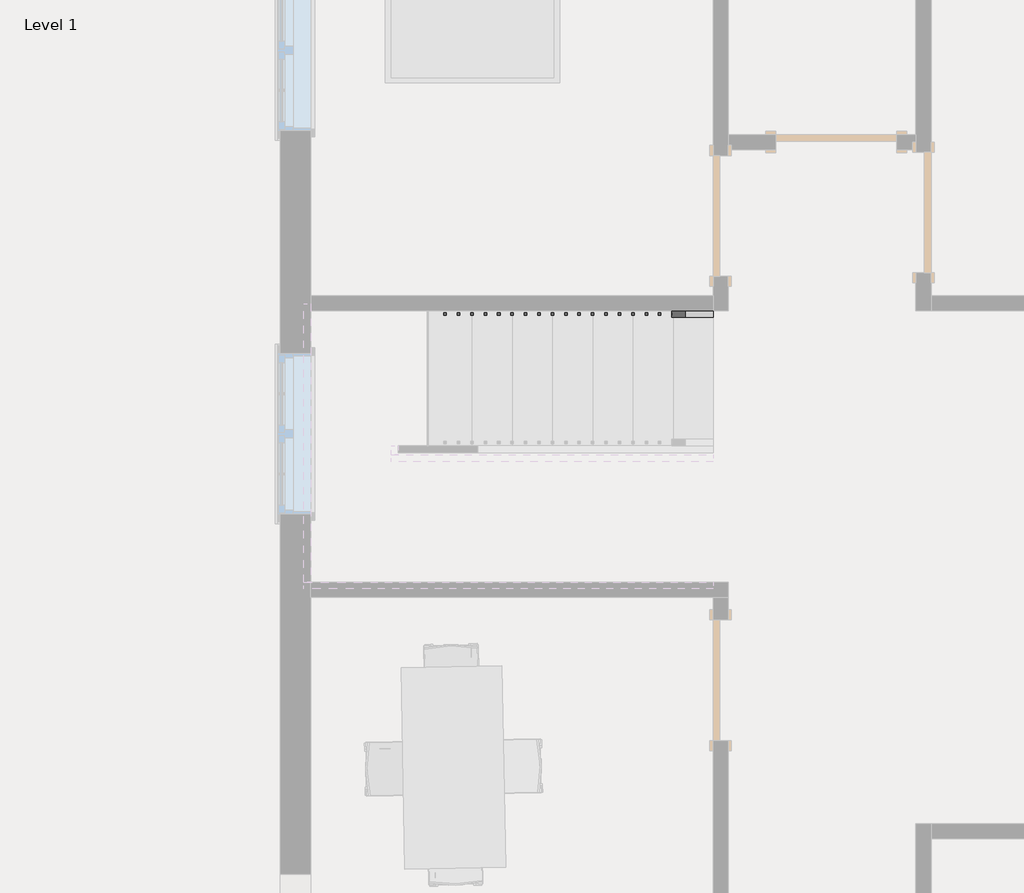
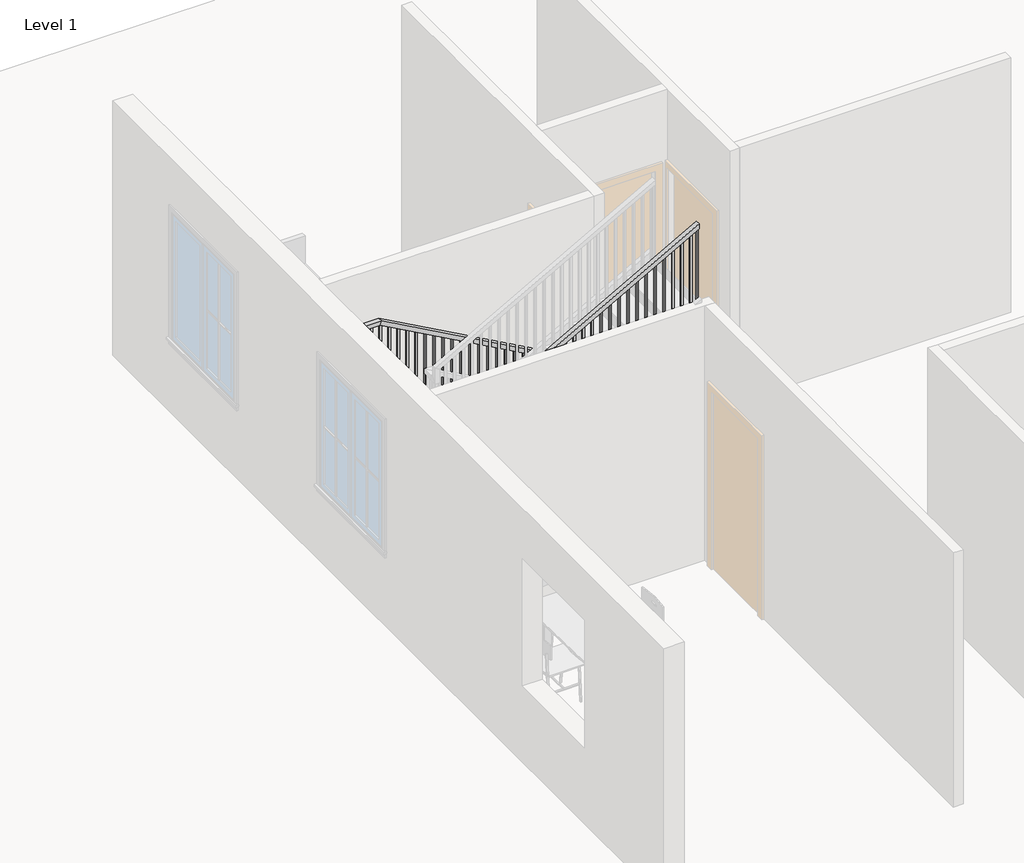
# One storey, part 2 of 3: 1 railing.
"""IFC4 building model written with IfcOpenShell, lengths in millimetres."""

from ifc_helpers import new_model, si_unit, frame, origin, place, context, project, spatial, polyline, outline, extrude, faceted_brep, element, save

model = new_model("IFC4")

# Units and contexts
model_context = context("Model", 3, world=origin())
ifc_project = project(units=[si_unit("LENGTHUNIT", "METRE", prefix="MILLI")], contexts=[model_context])

# Site, building, storey
site = spatial("IfcSite", under=ifc_project)
building = spatial("IfcBuilding", under=site)
storey = spatial("IfcBuildingStorey", under=building, Name="Level 1", Elevation=0.0)

# Railing
placement = place(None, origin())
element("IfcRailing", 1, ObjectType="Handrail - Rectangular", at=placement, inside=storey, context=model_context, shape_type="SolidModel", body=[
    faceted_brep([(4295.1355783, 9918.7, 1083.7333333), (4295.1355783, 9918.7, 1025.620221), (4295.1355783, 9969.5, 1025.620221), (4295.1355783, 9969.5, 1083.7333333), (1856.7355783, 9918.7, 2438.4), (1843.5719761, 9918.7, 2387.6), (1843.5719761, 9969.5, 2387.6), (1856.7355783, 9969.5, 2438.4), (1295.4, 9918.7, 2438.4), (1295.4, 9918.7, 2387.6), (1244.6, 9969.5, 2387.6), (1244.6, 9969.5, 2438.4), (1295.4, 7962.9, 2438.4), (1295.4, 7962.9, 2387.6), (1244.6, 7912.1, 2387.6), (1244.6, 7912.1, 2438.4), (1551.9355783, 7962.9, 2438.4), (1565.0991806, 7962.9, 2387.6), (1565.0991806, 7912.1, 2387.6), (1551.9355783, 7912.1, 2438.4), (4295.1355783, 7962.9, 3962.4), (4295.1355783, 7912.1, 3962.4), (4295.1355783, 7912.1, 3904.2868876), (4295.1355783, 7962.9, 3904.2868876)], [[[0, 1, 2, 3]], [[1, 0, 4, 5]], [[2, 1, 5, 6]], [[3, 2, 6, 7]], [[0, 3, 7, 4]], [[5, 4, 8, 9]], [[6, 5, 9, 10]], [[7, 6, 10, 11]], [[4, 7, 11, 8]], [[9, 8, 12, 13]], [[10, 9, 13, 14]], [[11, 10, 14, 15]], [[8, 11, 15, 12]], [[13, 12, 16, 17]], [[14, 13, 17, 18]], [[15, 14, 18, 19]], [[12, 15, 19, 16]], [[20, 21, 22, 23]], [[17, 16, 20, 23]], [[18, 17, 23, 22]], [[19, 18, 22, 21]], [[16, 19, 21, 20]]]),
    extrude(outline(polyline([(3865.8365664, 4225.925), (3855.253233, 4206.875), (2878.6666667, 4206.875), (2878.6666667, 4225.925), (3865.8365664, 4225.925)])), frame((0.0, 7927.975, 0.0), z_axis=(0.0, 1.0, 0.0), x_axis=(0.0, 0.0, 1.0)), (0.0, 0.0, 1.0), 19.05),
    extrude(outline(polyline([(3809.3921219, 4124.325), (3798.8087886, 4105.275), (2878.6666667, 4105.275), (2878.6666667, 4124.325), (3809.3921219, 4124.325)])), frame((0.0, 7927.975, 0.0), z_axis=(0.0, 1.0, 0.0), x_axis=(0.0, 0.0, 1.0)), (0.0, 0.0, 1.0), 19.05),
    extrude(outline(polyline([(3752.9476775, 4022.725), (3742.3643441, 4003.675), (2878.6666667, 4003.675), (2878.6666667, 4022.725), (3752.9476775, 4022.725)])), frame((0.0, 7927.975, 0.0), z_axis=(0.0, 1.0, 0.0), x_axis=(0.0, 0.0, 1.0)), (0.0, 0.0, 1.0), 19.05),
    extrude(outline(polyline([(3696.503233, 3921.125), (3685.9198997, 3902.075), (2709.3333333, 3902.075), (2709.3333333, 3921.125), (3696.503233, 3921.125)])), frame((0.0, 7927.975, 0.0), z_axis=(0.0, 1.0, 0.0), x_axis=(0.0, 0.0, 1.0)), (0.0, 0.0, 1.0), 19.05),
    extrude(outline(polyline([(3640.0587886, 3819.525), (3629.4754552, 3800.475), (2709.3333333, 3800.475), (2709.3333333, 3819.525), (3640.0587886, 3819.525)])), frame((0.0, 7927.975, 0.0), z_axis=(0.0, 1.0, 0.0), x_axis=(0.0, 0.0, 1.0)), (0.0, 0.0, 1.0), 19.05),
    extrude(outline(polyline([(3583.6143441, 3717.925), (3573.0310108, 3698.875), (2709.3333333, 3698.875), (2709.3333333, 3717.925), (3583.6143441, 3717.925)])), frame((0.0, 7927.975, 0.0), z_axis=(0.0, 1.0, 0.0), x_axis=(0.0, 0.0, 1.0)), (0.0, 0.0, 1.0), 19.05),
    extrude(outline(polyline([(3527.1698997, 3616.325), (3516.5865664, 3597.275), (2540.0, 3597.275), (2540.0, 3616.325), (3527.1698997, 3616.325)])), frame((0.0, 7927.975, 0.0), z_axis=(0.0, 1.0, 0.0), x_axis=(0.0, 0.0, 1.0)), (0.0, 0.0, 1.0), 19.05),
    extrude(outline(polyline([(3470.7254552, 3514.725), (3460.1421219, 3495.675), (2540.0, 3495.675), (2540.0, 3514.725), (3470.7254552, 3514.725)])), frame((0.0, 7927.975, 0.0), z_axis=(0.0, 1.0, 0.0), x_axis=(0.0, 0.0, 1.0)), (0.0, 0.0, 1.0), 19.05),
    extrude(outline(polyline([(3414.2810108, 3413.125), (3403.6976775, 3394.075), (2540.0, 3394.075), (2540.0, 3413.125), (3414.2810108, 3413.125)])), frame((0.0, 7927.975, 0.0), z_axis=(0.0, 1.0, 0.0), x_axis=(0.0, 0.0, 1.0)), (0.0, 0.0, 1.0), 19.05),
    extrude(outline(polyline([(3357.8365664, 3311.525), (3347.253233, 3292.475), (2370.6666667, 3292.475), (2370.6666667, 3311.525), (3357.8365664, 3311.525)])), frame((0.0, 7927.975, 0.0), z_axis=(0.0, 1.0, 0.0), x_axis=(0.0, 0.0, 1.0)), (0.0, 0.0, 1.0), 19.05),
    extrude(outline(polyline([(3301.3921219, 3209.925), (3290.8087886, 3190.875), (2370.6666667, 3190.875), (2370.6666667, 3209.925), (3301.3921219, 3209.925)])), frame((0.0, 7927.975, 0.0), z_axis=(0.0, 1.0, 0.0), x_axis=(0.0, 0.0, 1.0)), (0.0, 0.0, 1.0), 19.05),
    extrude(outline(polyline([(3244.9476775, 3108.325), (3234.3643441, 3089.275), (2370.6666667, 3089.275), (2370.6666667, 3108.325), (3244.9476775, 3108.325)])), frame((0.0, 7927.975, 0.0), z_axis=(0.0, 1.0, 0.0), x_axis=(0.0, 0.0, 1.0)), (0.0, 0.0, 1.0), 19.05),
    extrude(outline(polyline([(3188.503233, 3006.725), (3177.9198997, 2987.675), (2201.3333333, 2987.675), (2201.3333333, 3006.725), (3188.503233, 3006.725)])), frame((0.0, 7927.975, 0.0), z_axis=(0.0, 1.0, 0.0), x_axis=(0.0, 0.0, 1.0)), (0.0, 0.0, 1.0), 19.05),
    extrude(outline(polyline([(3132.0587886, 2905.125), (3121.4754552, 2886.075), (2201.3333333, 2886.075), (2201.3333333, 2905.125), (3132.0587886, 2905.125)])), frame((0.0, 7927.975, 0.0), z_axis=(0.0, 1.0, 0.0), x_axis=(0.0, 0.0, 1.0)), (0.0, 0.0, 1.0), 19.05),
    extrude(outline(polyline([(3075.6143441, 2803.525), (3065.0310108, 2784.475), (2201.3333333, 2784.475), (2201.3333333, 2803.525), (3075.6143441, 2803.525)])), frame((0.0, 7927.975, 0.0), z_axis=(0.0, 1.0, 0.0), x_axis=(0.0, 0.0, 1.0)), (0.0, 0.0, 1.0), 19.05),
    extrude(outline(polyline([(3019.1698997, 2701.925), (3008.5865664, 2682.875), (2032.0, 2682.875), (2032.0, 2701.925), (3019.1698997, 2701.925)])), frame((0.0, 7927.975, 0.0), z_axis=(0.0, 1.0, 0.0), x_axis=(0.0, 0.0, 1.0)), (0.0, 0.0, 1.0), 19.05),
    extrude(outline(polyline([(2962.7254552, 2600.325), (2952.1421219, 2581.275), (2032.0, 2581.275), (2032.0, 2600.325), (2962.7254552, 2600.325)])), frame((0.0, 7927.975, 0.0), z_axis=(0.0, 1.0, 0.0), x_axis=(0.0, 0.0, 1.0)), (0.0, 0.0, 1.0), 19.05),
    extrude(outline(polyline([(2906.2810108, 2498.725), (2895.6976775, 2479.675), (2032.0, 2479.675), (2032.0, 2498.725), (2906.2810108, 2498.725)])), frame((0.0, 7927.975, 0.0), z_axis=(0.0, 1.0, 0.0), x_axis=(0.0, 0.0, 1.0)), (0.0, 0.0, 1.0), 19.05),
    extrude(outline(polyline([(2849.8365664, 2397.125), (2839.253233, 2378.075), (1862.6666667, 2378.075), (1862.6666667, 2397.125), (2849.8365664, 2397.125)])), frame((0.0, 7927.975, 0.0), z_axis=(0.0, 1.0, 0.0), x_axis=(0.0, 0.0, 1.0)), (0.0, 0.0, 1.0), 19.05),
    extrude(outline(polyline([(2793.3921219, 2295.525), (2782.8087886, 2276.475), (1862.6666667, 2276.475), (1862.6666667, 2295.525), (2793.3921219, 2295.525)])), frame((0.0, 7927.975, 0.0), z_axis=(0.0, 1.0, 0.0), x_axis=(0.0, 0.0, 1.0)), (0.0, 0.0, 1.0), 19.05),
    extrude(outline(polyline([(2736.9476775, 2193.925), (2726.3643441, 2174.875), (1862.6666667, 2174.875), (1862.6666667, 2193.925), (2736.9476775, 2193.925)])), frame((0.0, 7927.975, 0.0), z_axis=(0.0, 1.0, 0.0), x_axis=(0.0, 0.0, 1.0)), (0.0, 0.0, 1.0), 19.05),
    extrude(outline(polyline([(2680.503233, 2092.325), (2669.9198997, 2073.275), (1693.3333333, 2073.275), (1693.3333333, 2092.325), (2680.503233, 2092.325)])), frame((0.0, 7927.975, 0.0), z_axis=(0.0, 1.0, 0.0), x_axis=(0.0, 0.0, 1.0)), (0.0, 0.0, 1.0), 19.05),
    extrude(outline(polyline([(2624.0587886, 1990.725), (2613.4754552, 1971.675), (1693.3333333, 1971.675), (1693.3333333, 1990.725), (2624.0587886, 1990.725)])), frame((0.0, 7927.975, 0.0), z_axis=(0.0, 1.0, 0.0), x_axis=(0.0, 0.0, 1.0)), (0.0, 0.0, 1.0), 19.05),
    extrude(outline(polyline([(2567.6143441, 1889.125), (2557.0310108, 1870.075), (1693.3333333, 1870.075), (1693.3333333, 1889.125), (2567.6143441, 1889.125)])), frame((0.0, 7927.975, 0.0), z_axis=(0.0, 1.0, 0.0), x_axis=(0.0, 0.0, 1.0)), (0.0, 0.0, 1.0), 19.05),
    extrude(outline(polyline([(2511.1698997, 1787.525), (2500.5865664, 1768.475), (1524.0, 1768.475), (1524.0, 1787.525), (2511.1698997, 1787.525)])), frame((0.0, 7927.975, 0.0), z_axis=(0.0, 1.0, 0.0), x_axis=(0.0, 0.0, 1.0)), (0.0, 0.0, 1.0), 19.05),
    extrude(outline(polyline([(2454.7254552, 1685.925), (2444.1421219, 1666.875), (1524.0, 1666.875), (1524.0, 1685.925), (2454.7254552, 1685.925)])), frame((0.0, 7927.975, 0.0), z_axis=(0.0, 1.0, 0.0), x_axis=(0.0, 0.0, 1.0)), (0.0, 0.0, 1.0), 19.05),
    extrude(outline(polyline([(2398.2810108, 1584.325), (2387.6976775, 1565.275), (1524.0, 1565.275), (1524.0, 1584.325), (2398.2810108, 1584.325)])), frame((0.0, 7927.975, 0.0), z_axis=(0.0, 1.0, 0.0), x_axis=(0.0, 0.0, 1.0)), (0.0, 0.0, 1.0), 19.05),
    extrude(outline(polyline([(1463.675, 7927.975), (1463.675, 7947.025), (1482.725, 7947.025), (1482.725, 7927.975), (1463.675, 7927.975)])), frame((0.0, 0.0, 1524.0), z_axis=(0.0, 0.0, 1.0), x_axis=(1.0, 0.0, 0.0)), (0.0, 0.0, 1.0), 863.6),
    extrude(outline(polyline([(1362.075, 7927.975), (1362.075, 7947.025), (1381.125, 7947.025), (1381.125, 7927.975), (1362.075, 7927.975)])), frame((0.0, 0.0, 1524.0), z_axis=(0.0, 0.0, 1.0), x_axis=(1.0, 0.0, 0.0)), (0.0, 0.0, 1.0), 863.6),
    extrude(outline(polyline([(1260.475, 8023.225), (1279.525, 8023.225), (1279.525, 8004.175), (1260.475, 8004.175), (1260.475, 8023.225)])), frame((0.0, 0.0, 1524.0), z_axis=(0.0, 0.0, 1.0), x_axis=(1.0, 0.0, 0.0)), (0.0, 0.0, 1.0), 863.6),
    extrude(outline(polyline([(1260.475, 8124.825), (1279.525, 8124.825), (1279.525, 8105.775), (1260.475, 8105.775), (1260.475, 8124.825)])), frame((0.0, 0.0, 1524.0), z_axis=(0.0, 0.0, 1.0), x_axis=(1.0, 0.0, 0.0)), (0.0, 0.0, 1.0), 863.6),
    extrude(outline(polyline([(1260.475, 8226.425), (1279.525, 8226.425), (1279.525, 8207.375), (1260.475, 8207.375), (1260.475, 8226.425)])), frame((0.0, 0.0, 1524.0), z_axis=(0.0, 0.0, 1.0), x_axis=(1.0, 0.0, 0.0)), (0.0, 0.0, 1.0), 863.6),
    extrude(outline(polyline([(1260.475, 8328.025), (1279.525, 8328.025), (1279.525, 8308.975), (1260.475, 8308.975), (1260.475, 8328.025)])), frame((0.0, 0.0, 1524.0), z_axis=(0.0, 0.0, 1.0), x_axis=(1.0, 0.0, 0.0)), (0.0, 0.0, 1.0), 863.6),
    extrude(outline(polyline([(1260.475, 8429.625), (1279.525, 8429.625), (1279.525, 8410.575), (1260.475, 8410.575), (1260.475, 8429.625)])), frame((0.0, 0.0, 1524.0), z_axis=(0.0, 0.0, 1.0), x_axis=(1.0, 0.0, 0.0)), (0.0, 0.0, 1.0), 863.6),
    extrude(outline(polyline([(1260.475, 8531.225), (1279.525, 8531.225), (1279.525, 8512.175), (1260.475, 8512.175), (1260.475, 8531.225)])), frame((0.0, 0.0, 1524.0), z_axis=(0.0, 0.0, 1.0), x_axis=(1.0, 0.0, 0.0)), (0.0, 0.0, 1.0), 863.6),
    extrude(outline(polyline([(1260.475, 8632.825), (1279.525, 8632.825), (1279.525, 8613.775), (1260.475, 8613.775), (1260.475, 8632.825)])), frame((0.0, 0.0, 1524.0), z_axis=(0.0, 0.0, 1.0), x_axis=(1.0, 0.0, 0.0)), (0.0, 0.0, 1.0), 863.6),
    extrude(outline(polyline([(1260.475, 8734.425), (1279.525, 8734.425), (1279.525, 8715.375), (1260.475, 8715.375), (1260.475, 8734.425)])), frame((0.0, 0.0, 1524.0), z_axis=(0.0, 0.0, 1.0), x_axis=(1.0, 0.0, 0.0)), (0.0, 0.0, 1.0), 863.6),
    extrude(outline(polyline([(1260.475, 8836.025), (1279.525, 8836.025), (1279.525, 8816.975), (1260.475, 8816.975), (1260.475, 8836.025)])), frame((0.0, 0.0, 1524.0), z_axis=(0.0, 0.0, 1.0), x_axis=(1.0, 0.0, 0.0)), (0.0, 0.0, 1.0), 863.6),
    extrude(outline(polyline([(1260.475, 8937.625), (1279.525, 8937.625), (1279.525, 8918.575), (1260.475, 8918.575), (1260.475, 8937.625)])), frame((0.0, 0.0, 1524.0), z_axis=(0.0, 0.0, 1.0), x_axis=(1.0, 0.0, 0.0)), (0.0, 0.0, 1.0), 863.6),
    extrude(outline(polyline([(1260.475, 9039.225), (1279.525, 9039.225), (1279.525, 9020.175), (1260.475, 9020.175), (1260.475, 9039.225)])), frame((0.0, 0.0, 1524.0), z_axis=(0.0, 0.0, 1.0), x_axis=(1.0, 0.0, 0.0)), (0.0, 0.0, 1.0), 863.6),
    extrude(outline(polyline([(1260.475, 9140.825), (1279.525, 9140.825), (1279.525, 9121.775), (1260.475, 9121.775), (1260.475, 9140.825)])), frame((0.0, 0.0, 1524.0), z_axis=(0.0, 0.0, 1.0), x_axis=(1.0, 0.0, 0.0)), (0.0, 0.0, 1.0), 863.6),
    extrude(outline(polyline([(1260.475, 9242.425), (1279.525, 9242.425), (1279.525, 9223.375), (1260.475, 9223.375), (1260.475, 9242.425)])), frame((0.0, 0.0, 1524.0), z_axis=(0.0, 0.0, 1.0), x_axis=(1.0, 0.0, 0.0)), (0.0, 0.0, 1.0), 863.6),
    extrude(outline(polyline([(1260.475, 9344.025), (1279.525, 9344.025), (1279.525, 9324.975), (1260.475, 9324.975), (1260.475, 9344.025)])), frame((0.0, 0.0, 1524.0), z_axis=(0.0, 0.0, 1.0), x_axis=(1.0, 0.0, 0.0)), (0.0, 0.0, 1.0), 863.6),
    extrude(outline(polyline([(1260.475, 9445.625), (1279.525, 9445.625), (1279.525, 9426.575), (1260.475, 9426.575), (1260.475, 9445.625)])), frame((0.0, 0.0, 1524.0), z_axis=(0.0, 0.0, 1.0), x_axis=(1.0, 0.0, 0.0)), (0.0, 0.0, 1.0), 863.6),
    extrude(outline(polyline([(1260.475, 9547.225), (1279.525, 9547.225), (1279.525, 9528.175), (1260.475, 9528.175), (1260.475, 9547.225)])), frame((0.0, 0.0, 1524.0), z_axis=(0.0, 0.0, 1.0), x_axis=(1.0, 0.0, 0.0)), (0.0, 0.0, 1.0), 863.6),
    extrude(outline(polyline([(1260.475, 9648.825), (1279.525, 9648.825), (1279.525, 9629.775), (1260.475, 9629.775), (1260.475, 9648.825)])), frame((0.0, 0.0, 1524.0), z_axis=(0.0, 0.0, 1.0), x_axis=(1.0, 0.0, 0.0)), (0.0, 0.0, 1.0), 863.6),
    extrude(outline(polyline([(1260.475, 9750.425), (1279.525, 9750.425), (1279.525, 9731.375), (1260.475, 9731.375), (1260.475, 9750.425)])), frame((0.0, 0.0, 1524.0), z_axis=(0.0, 0.0, 1.0), x_axis=(1.0, 0.0, 0.0)), (0.0, 0.0, 1.0), 863.6),
    extrude(outline(polyline([(1260.475, 9852.025), (1279.525, 9852.025), (1279.525, 9832.975), (1260.475, 9832.975), (1260.475, 9852.025)])), frame((0.0, 0.0, 1524.0), z_axis=(0.0, 0.0, 1.0), x_axis=(1.0, 0.0, 0.0)), (0.0, 0.0, 1.0), 863.6),
    extrude(outline(polyline([(1358.2605783, 9953.625), (1358.2605783, 9934.575), (1339.2105783, 9934.575), (1339.2105783, 9953.625), (1358.2605783, 9953.625)])), frame((0.0, 0.0, 1524.0), z_axis=(0.0, 0.0, 1.0), x_axis=(1.0, 0.0, 0.0)), (0.0, 0.0, 1.0), 863.6),
    extrude(outline(polyline([(1459.8605783, 9953.625), (1459.8605783, 9934.575), (1440.8105783, 9934.575), (1440.8105783, 9953.625), (1459.8605783, 9953.625)])), frame((0.0, 0.0, 1524.0), z_axis=(0.0, 0.0, 1.0), x_axis=(1.0, 0.0, 0.0)), (0.0, 0.0, 1.0), 863.6),
    extrude(outline(polyline([(1561.4605783, 9953.625), (1561.4605783, 9934.575), (1542.4105783, 9934.575), (1542.4105783, 9953.625), (1561.4605783, 9953.625)])), frame((0.0, 0.0, 1524.0), z_axis=(0.0, 0.0, 1.0), x_axis=(1.0, 0.0, 0.0)), (0.0, 0.0, 1.0), 863.6),
    extrude(outline(polyline([(1663.0605783, 9953.625), (1663.0605783, 9934.575), (1644.0105783, 9934.575), (1644.0105783, 9953.625), (1663.0605783, 9953.625)])), frame((0.0, 0.0, 1524.0), z_axis=(0.0, 0.0, 1.0), x_axis=(1.0, 0.0, 0.0)), (0.0, 0.0, 1.0), 863.6),
    extrude(outline(polyline([(1764.6605783, 9953.625), (1764.6605783, 9934.575), (1745.6105783, 9934.575), (1745.6105783, 9953.625), (1764.6605783, 9953.625)])), frame((0.0, 0.0, 1524.0), z_axis=(0.0, 0.0, 1.0), x_axis=(1.0, 0.0, 0.0)), (0.0, 0.0, 1.0), 863.6),
    extrude(outline(polyline([(2374.995221, 1866.2605783), (2385.5785543, 1847.2105783), (1524.0, 1847.2105783), (1524.0, 1866.2605783), (2374.995221, 1866.2605783)])), frame((0.0, 9934.575, 0.0), z_axis=(0.0, 1.0, 0.0), x_axis=(0.0, 0.0, 1.0)), (0.0, 0.0, 1.0), 19.05),
    extrude(outline(polyline([(2318.5507765, 1967.8605783), (2329.1341099, 1948.8105783), (1354.6666667, 1948.8105783), (1354.6666667, 1967.8605783), (2318.5507765, 1967.8605783)])), frame((0.0, 9934.575, 0.0), z_axis=(0.0, 1.0, 0.0), x_axis=(0.0, 0.0, 1.0)), (0.0, 0.0, 1.0), 19.05),
    extrude(outline(polyline([(2262.1063321, 2069.4605783), (2272.6896654, 2050.4105783), (1354.6666667, 2050.4105783), (1354.6666667, 2069.4605783), (2262.1063321, 2069.4605783)])), frame((0.0, 9934.575, 0.0), z_axis=(0.0, 1.0, 0.0), x_axis=(0.0, 0.0, 1.0)), (0.0, 0.0, 1.0), 19.05),
    extrude(outline(polyline([(2205.6618876, 2171.0605783), (2216.245221, 2152.0105783), (1354.6666667, 2152.0105783), (1354.6666667, 2171.0605783), (2205.6618876, 2171.0605783)])), frame((0.0, 9934.575, 0.0), z_axis=(0.0, 1.0, 0.0), x_axis=(0.0, 0.0, 1.0)), (0.0, 0.0, 1.0), 19.05),
    extrude(outline(polyline([(2149.2174432, 2272.6605783), (2159.8007765, 2253.6105783), (1185.3333333, 2253.6105783), (1185.3333333, 2272.6605783), (2149.2174432, 2272.6605783)])), frame((0.0, 9934.575, 0.0), z_axis=(0.0, 1.0, 0.0), x_axis=(0.0, 0.0, 1.0)), (0.0, 0.0, 1.0), 19.05),
    extrude(outline(polyline([(2092.7729988, 2374.2605783), (2103.3563321, 2355.2105783), (1185.3333333, 2355.2105783), (1185.3333333, 2374.2605783), (2092.7729988, 2374.2605783)])), frame((0.0, 9934.575, 0.0), z_axis=(0.0, 1.0, 0.0), x_axis=(0.0, 0.0, 1.0)), (0.0, 0.0, 1.0), 19.05),
    extrude(outline(polyline([(2036.3285543, 2475.8605783), (2046.9118876, 2456.8105783), (1185.3333333, 2456.8105783), (1185.3333333, 2475.8605783), (2036.3285543, 2475.8605783)])), frame((0.0, 9934.575, 0.0), z_axis=(0.0, 1.0, 0.0), x_axis=(0.0, 0.0, 1.0)), (0.0, 0.0, 1.0), 19.05),
    extrude(outline(polyline([(1979.8841099, 2577.4605783), (1990.4674432, 2558.4105783), (1016.0, 2558.4105783), (1016.0, 2577.4605783), (1979.8841099, 2577.4605783)])), frame((0.0, 9934.575, 0.0), z_axis=(0.0, 1.0, 0.0), x_axis=(0.0, 0.0, 1.0)), (0.0, 0.0, 1.0), 19.05),
    extrude(outline(polyline([(1923.4396654, 2679.0605783), (1934.0229988, 2660.0105783), (1016.0, 2660.0105783), (1016.0, 2679.0605783), (1923.4396654, 2679.0605783)])), frame((0.0, 9934.575, 0.0), z_axis=(0.0, 1.0, 0.0), x_axis=(0.0, 0.0, 1.0)), (0.0, 0.0, 1.0), 19.05),
    extrude(outline(polyline([(1866.995221, 2780.6605783), (1877.5785543, 2761.6105783), (1016.0, 2761.6105783), (1016.0, 2780.6605783), (1866.995221, 2780.6605783)])), frame((0.0, 9934.575, 0.0), z_axis=(0.0, 1.0, 0.0), x_axis=(0.0, 0.0, 1.0)), (0.0, 0.0, 1.0), 19.05),
    extrude(outline(polyline([(1810.5507765, 2882.2605783), (1821.1341099, 2863.2105783), (846.6666667, 2863.2105783), (846.6666667, 2882.2605783), (1810.5507765, 2882.2605783)])), frame((0.0, 9934.575, 0.0), z_axis=(0.0, 1.0, 0.0), x_axis=(0.0, 0.0, 1.0)), (0.0, 0.0, 1.0), 19.05),
    extrude(outline(polyline([(1754.1063321, 2983.8605783), (1764.6896654, 2964.8105783), (846.6666667, 2964.8105783), (846.6666667, 2983.8605783), (1754.1063321, 2983.8605783)])), frame((0.0, 9934.575, 0.0), z_axis=(0.0, 1.0, 0.0), x_axis=(0.0, 0.0, 1.0)), (0.0, 0.0, 1.0), 19.05),
    extrude(outline(polyline([(1697.6618876, 3085.4605783), (1708.245221, 3066.4105783), (846.6666667, 3066.4105783), (846.6666667, 3085.4605783), (1697.6618876, 3085.4605783)])), frame((0.0, 9934.575, 0.0), z_axis=(0.0, 1.0, 0.0), x_axis=(0.0, 0.0, 1.0)), (0.0, 0.0, 1.0), 19.05),
    extrude(outline(polyline([(1641.2174432, 3187.0605783), (1651.8007765, 3168.0105783), (677.3333333, 3168.0105783), (677.3333333, 3187.0605783), (1641.2174432, 3187.0605783)])), frame((0.0, 9934.575, 0.0), z_axis=(0.0, 1.0, 0.0), x_axis=(0.0, 0.0, 1.0)), (0.0, 0.0, 1.0), 19.05),
    extrude(outline(polyline([(1584.7729988, 3288.6605783), (1595.3563321, 3269.6105783), (677.3333333, 3269.6105783), (677.3333333, 3288.6605783), (1584.7729988, 3288.6605783)])), frame((0.0, 9934.575, 0.0), z_axis=(0.0, 1.0, 0.0), x_axis=(0.0, 0.0, 1.0)), (0.0, 0.0, 1.0), 19.05),
    extrude(outline(polyline([(1528.3285543, 3390.2605783), (1538.9118876, 3371.2105783), (677.3333333, 3371.2105783), (677.3333333, 3390.2605783), (1528.3285543, 3390.2605783)])), frame((0.0, 9934.575, 0.0), z_axis=(0.0, 1.0, 0.0), x_axis=(0.0, 0.0, 1.0)), (0.0, 0.0, 1.0), 19.05),
    extrude(outline(polyline([(1471.8841099, 3491.8605783), (1482.4674432, 3472.8105783), (508.0, 3472.8105783), (508.0, 3491.8605783), (1471.8841099, 3491.8605783)])), frame((0.0, 9934.575, 0.0), z_axis=(0.0, 1.0, 0.0), x_axis=(0.0, 0.0, 1.0)), (0.0, 0.0, 1.0), 19.05),
    extrude(outline(polyline([(1415.4396654, 3593.4605783), (1426.0229988, 3574.4105783), (508.0, 3574.4105783), (508.0, 3593.4605783), (1415.4396654, 3593.4605783)])), frame((0.0, 9934.575, 0.0), z_axis=(0.0, 1.0, 0.0), x_axis=(0.0, 0.0, 1.0)), (0.0, 0.0, 1.0), 19.05),
    extrude(outline(polyline([(1358.995221, 3695.0605783), (1369.5785543, 3676.0105783), (508.0, 3676.0105783), (508.0, 3695.0605783), (1358.995221, 3695.0605783)])), frame((0.0, 9934.575, 0.0), z_axis=(0.0, 1.0, 0.0), x_axis=(0.0, 0.0, 1.0)), (0.0, 0.0, 1.0), 19.05),
    extrude(outline(polyline([(1302.5507765, 3796.6605783), (1313.1341099, 3777.6105783), (338.6666667, 3777.6105783), (338.6666667, 3796.6605783), (1302.5507765, 3796.6605783)])), frame((0.0, 9934.575, 0.0), z_axis=(0.0, 1.0, 0.0), x_axis=(0.0, 0.0, 1.0)), (0.0, 0.0, 1.0), 19.05),
    extrude(outline(polyline([(1246.1063321, 3898.2605783), (1256.6896654, 3879.2105783), (338.6666667, 3879.2105783), (338.6666667, 3898.2605783), (1246.1063321, 3898.2605783)])), frame((0.0, 9934.575, 0.0), z_axis=(0.0, 1.0, 0.0), x_axis=(0.0, 0.0, 1.0)), (0.0, 0.0, 1.0), 19.05),
    extrude(outline(polyline([(1189.6618876, 3999.8605783), (1200.245221, 3980.8105783), (338.6666667, 3980.8105783), (338.6666667, 3999.8605783), (1189.6618876, 3999.8605783)])), frame((0.0, 9934.575, 0.0), z_axis=(0.0, 1.0, 0.0), x_axis=(0.0, 0.0, 1.0)), (0.0, 0.0, 1.0), 19.05),
    extrude(outline(polyline([(1133.2174432, 4101.4605783), (1143.8007765, 4082.4105783), (169.3333333, 4082.4105783), (169.3333333, 4101.4605783), (1133.2174432, 4101.4605783)])), frame((0.0, 9934.575, 0.0), z_axis=(0.0, 1.0, 0.0), x_axis=(0.0, 0.0, 1.0)), (0.0, 0.0, 1.0), 19.05),
    extrude(outline(polyline([(1076.7729988, 4203.0605783), (1087.3563321, 4184.0105783), (169.3333333, 4184.0105783), (169.3333333, 4203.0605783), (1076.7729988, 4203.0605783)])), frame((0.0, 9934.575, 0.0), z_axis=(0.0, 1.0, 0.0), x_axis=(0.0, 0.0, 1.0)), (0.0, 0.0, 1.0), 19.05),
    extrude(outline(polyline([(1260.475, 7947.025), (1279.525, 7947.025), (1279.525, 7927.975), (1260.475, 7927.975), (1260.475, 7947.025)])), frame((0.0, 0.0, 1524.0), z_axis=(0.0, 0.0, 1.0), x_axis=(1.0, 0.0, 0.0)), (0.0, 0.0, 1.0), 863.6),
    extrude(outline(polyline([(1279.525, 9953.625), (1279.525, 9934.575), (1260.475, 9934.575), (1260.475, 9953.625), (1279.525, 9953.625)])), frame((0.0, 0.0, 1524.0), z_axis=(0.0, 0.0, 1.0), x_axis=(1.0, 0.0, 0.0)), (0.0, 0.0, 1.0), 863.6),
    extrude(outline(polyline([(3904.2868876, 4295.1355783), (3893.7035543, 4276.0855783), (2878.6666667, 4276.0855783), (2878.6666667, 4295.1355783), (3904.2868876, 4295.1355783)])), frame((0.0, 7927.975, 0.0), z_axis=(0.0, 1.0, 0.0), x_axis=(0.0, 0.0, 1.0)), (0.0, 0.0, 1.0), 19.05),
    extrude(outline(polyline([(1025.620221, 4295.1355783), (1036.2035543, 4276.0855783), (169.3333333, 4276.0855783), (169.3333333, 4295.1355783), (1025.620221, 4295.1355783)])), frame((0.0, 9934.575, 0.0), z_axis=(0.0, 1.0, 0.0), x_axis=(0.0, 0.0, 1.0)), (0.0, 0.0, 1.0), 19.05),
])

save(model, "model.ifc")

# Revit data of these elements
# Type "Handrail - Rectangular"
#   Assembly Code = "C2010400"
#   built-in parameter 1008612 = 0.0416667 (stored number, unit not read)
#   built-in parameter 1008611 = 0.0416667 (stored number, unit not read)
#   built-in parameter 1008609 = 0.333333 (stored number, unit not read)
#   built-in parameter 1008604 = 0.166667 (stored number, unit not read)
#   built-in parameter 1008603 = 0.166667 (stored number, unit not read)
#   Railing Height = 3' - 0"
#   built-in parameter 1008630 = 2
#   built-in parameter 1008610 = 2
#   built-in parameter 1008618 = Baluster - Square : 3/4"
# Element 1 (IfcRailing, "Handrail - Rectangular")
#   Phase Created = New Construction
